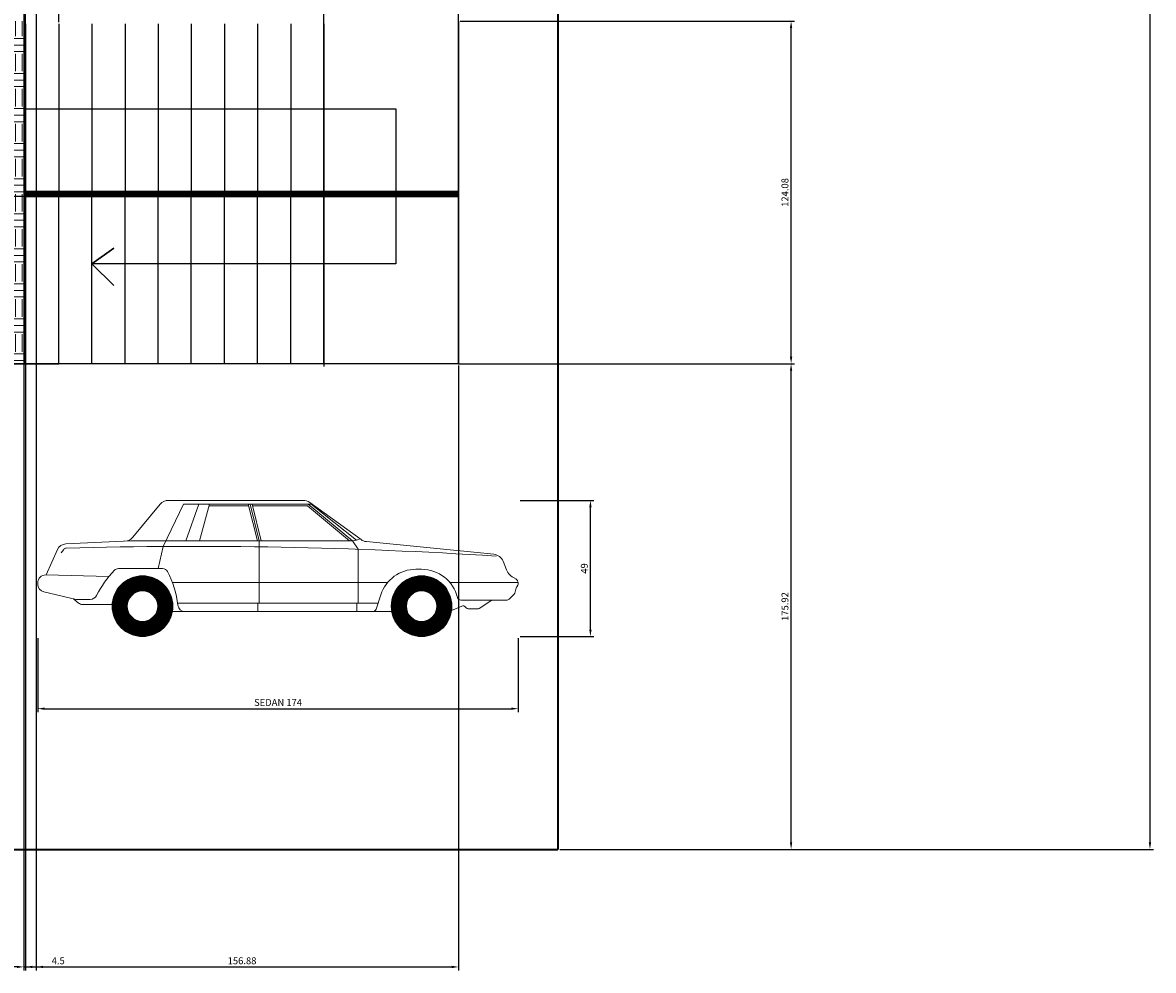
# Model space of a CAD drawing. Units: inches. Extents: x 204 to 942, y 1794 to 2670.
# Tile 2 of 6: x 533 to 942, y 1794 to 2138. Entities that reach past the tile are written whole.
import ezdxf

# ---------------------------------------------------------------- set-up
doc = ezdxf.new("R2010")
doc.units = ezdxf.units.IN
for name, color, linetype, lineweight in [('A-ANNO-DIMS', 2, 'Continuous', 18), ('A-FLOR-OTLN', 7, 'Continuous', 25), ('A-FLOR-STRS', 7, 'Continuous', 25), ('C-PRKG', 8, 'Continuous', 25), ('C-PRKG-VEHI', 8, 'Continuous', 18), ('C-PROP', 7, 'Continuous', 35)]:
    doc.layers.add(name, color=color, linetype=linetype, lineweight=lineweight)
doc.layers.add('A-FLOR-PATT', color=251, linetype='Continuous', lineweight=13, true_color=0x636466)
doc.styles.get("Standard").update_dxf_attribs({"font": 'arial.ttf'})
doc.dimstyles.new('ISO-25', dxfattribs={"dimtxt": 2.5, "dimasz": 2.5, "dimexe": 1.25, "dimexo": 0.625, "dimtad": 1, "dimtxsty": 'Standard', "dimcen": 2.5, "dimadec": 0, "dimazin": 0, "dimtfac": 1, "dimtmove": 0, "dimatfit": 3, "dimfxl": 1, "dimarcsym": 0})

# ---------------------------------------------------------------- blocks, each defined once
blk = doc.blocks.new('Car - sedan  side')
for p, q in [((-77.81, 49.34), (-126.58, 49.34)), ((-139.53, 35.99), (-129.64, 47.91)), ((-128.57, 32.64), (-121.22, 48.02)), ((-74.7, 48.02), (-121.22, 48.02)), ((-120.32, 34.67), (-115.67, 48.02)), ((-115.4, 34.67), (-111.74, 48.02)), ((-97.55, 47.3), (-111.94, 47.3)), ((-94.41, 34.67), (-97.73, 48.02)), ((-93.72, 34.67), (-97.04, 48.02)), ((-93.03, 34.67), (-96.34, 48.02)), ((-76.26, 47.3), (-96.16, 47.3)), ((-61.08, 34.66), (-76.26, 47.3)), ((-60.02, 34.65), (-76.07, 48.02)), ((-56.87, 35.13), (-75.48, 48.59)), ((-58.54, 34.93), (-74.99, 48.02)), ((-140.23, 34.67), (-163.88, 33.56)), ((-62.28, 34.67), (-140.23, 34.67)), ((-93.72, 19.62), (-93.72, 34.67)), ((-62.28, 34.67), (-60.02, 34.65)), ((-60.02, 34.65), (-58.54, 34.93)), ((-57.97, 31.61), (-60.02, 34.65)), ((-57.21, 35.38), (-58.54, 34.93)), ((-54.93, 34.4), (-8.75, 29.8)), ((-170.93, 22.32), (-166.81, 31.56)), ((-164.57, 31.6), (-165.48, 30.35)), ((-130.39, 24.63), (-128.57, 32.64)), ((-57.97, 19.62), (-57.97, 31.61)), ((-128.78, 24.63), (-144.79, 24.63)), ((-4.21, 24.18), (-5.42, 27.27)), ((-148.26, 21.7), (-171.11, 22.33)), ((-36.97, 24.38), (-34.94, 24.38)), ((-174, 19.51), (-174, 18.91)), ((-47.2, 19.62), (-125.23, 19.62)), ((-93.72, 12.14), (-93.72, 19.62)), ((-57.97, 12.14), (-57.97, 19.62)), ((0, 19.62), (-24.7, 19.62)), ((-160.12, 13.48), (-171.81, 16.16)), ((-159.22, 12.14), (-161.08, 13.7)), ((-155.01, 13.48), (-160.12, 13.48)), ((-51.4, 9.89), (-49.69, 15.14)), ((-4.23, 13.19), (-20.72, 13.19)), ((-9.5, 13.19), (-14.1, 10.2)), ((-3.22, 13.59), (-1.77, 14.97)), ((-147.03, 11.6), (-157.73, 11.6)), ((-120.62, 9.03), (-125.23, 9.03)), ((-50.67, 12.14), (-123.32, 12.14)), ((-45.76, 9.03), (-120.62, 9.03)), ((-94.21, 9.03), (-94.21, 12.14)), ((-58.39, 9.03), (-58.39, 12.14)), ((-20.36, 11.06), (-24.06, 9.44)), ((-18.83, 10.42), (-19.11, 10.76)), ((-14.68, 10.03), (-18.01, 10.03))]:
    blk.add_line(p, q)
at = {"const_width": 5.49}
for points in [[(-127.8, 11, -1), (-144.3, 11, -1)], [(-26.69, 11, -1), (-43.19, 11, -1)]]:
    blk.add_lwpolyline(points, format="xyb", close=True, dxfattribs=at)
for centre, radius in [((-136.05, 11), 11), ((-34.94, 11), 11), ((-136.05, 11), 5.51), ((-34.94, 11), 5.51)]:
    blk.add_circle(centre, radius)
for centre, radius, start, end in [((-126.58, 45.38), 3.97, 90, 140.3029), ((-77.81, 45.38), 3.97, 54.135, 90), ((-163.72, 30.18), 3.38, 92.6827, 155.9736), ((-142.58, 38.53), 3.97, 272.6827, 320.3029), ((-54.54, 38.35), 3.97, 234.135, 264.3123), ((-163.62, 30.91), 1.17, 91.491, 143.9553), ((-118.51, -1702.12), 1734.79, 86.34698, 91.49105), ((-9.15, 25.82), 4, 21.3107, 84.3123), ((-144.79, 22.64), 1.98, 90, 136.3964), ((-128.78, 22.64), 1.98, 28.1371, 90), ((-171.18, 19.51), 2.82, 88.4193, 180), ((-118.09, -2.78), 38.85, 136.3964, 152.9097), ((-157.14, 7.48), 34.14, 6.5135, 28.1371), ((-36.97, 11), 13.38, 90, 161.9732), ((-34.94, 11), 13.38, 13.5864, 90), ((0.9, 26.18), 5.49, 201.3107, 247.7048), ((-1.92, 19.3), 1.94, 325.3744, 67.7048), ((-171.18, 18.91), 2.82, 180, 257.0905), ((-3.82, 17.12), 2.96, 313.7173, 352.3839), ((2.46, 16.28), 3.37, 145.3744, 172.3839), ((-155.01, 16.1), 2.62, 270, 332.9097), ((-20.72, 14.43), 1.24, 193.5864, 270), ((-4.23, 14.65), 1.46, 270, 313.7173), ((-157.73, 13.93), 2.32, 230.1291, 270), ((-120.62, 11.65), 2.62, 186.5135, 270), ((-52.58, 10.27), 1.24, 270, 341.9732), ((-19.93, 10.09), 1.06, 39.301, 113.7159), ((-18.01, 11.09), 1.06, 219.301, 270), ((-14.68, 11.09), 1.06, 270, 303.047)]:
    blk.add_arc(centre, radius, start, end)
blk = doc.blocks.new('*D12')
at = {"layer": 'A-ANNO-DIMS', "color": 0, "lineweight": -2, "transparency": 16777216}
for p, q in [((727.37, 2624.26), (942.46, 2624.26)), ((941.21, 2621.76), (941.21, 1840.76)), ((727.37, 1838.26), (942.46, 1838.26))]:
    blk.add_line(p, q, dxfattribs=at)
at = {"layer": 'A-ANNO-DIMS', "color": 0, "transparency": 16777216}
for points in [[(940.79, 2621.76), (941.63, 2621.76), (941.21, 2624.26)], [(940.79, 1840.76), (941.63, 1840.76), (941.21, 1838.26)]]:
    blk.add_solid(points, dxfattribs=at)
at = {"layer": 'Defpoints', "color": 0, "transparency": 16777216}
for p in [(726.74, 2624.26), (726.74, 1838.26), (941.21, 1838.26)]:
    blk.add_point(p, dxfattribs=at)
at = {"layer": 'A-ANNO-DIMS', "color": 0, "transparency": 16777216, "insert": (939.31, 2231.26), "char_height": 2.5, "attachment_point": 5, "rotation": 90}
blk.add_mtext('786', dxfattribs=at)
blk = doc.blocks.new('*D36')
at = {"layer": 'A-ANNO-DIMS', "color": 0, "lineweight": -2, "transparency": 16777216}
for p, q in [((538.28, 1914.72), (538.28, 1887.97)), ((712.39, 1914.72), (712.39, 1887.97)), ((540.78, 1889.22), (709.89, 1889.22))]:
    blk.add_line(p, q, dxfattribs=at)
at = {"layer": 'A-ANNO-DIMS', "color": 0, "transparency": 16777216}
for points in [[(540.78, 1889.64), (540.78, 1888.81), (538.28, 1889.22)], [(709.89, 1889.64), (709.89, 1888.81), (712.39, 1889.22)]]:
    blk.add_solid(points, dxfattribs=at)
at = {"layer": 'Defpoints', "color": 0, "transparency": 16777216}
for p in [(538.28, 1915.34), (712.39, 1915.34), (712.39, 1889.22)]:
    blk.add_point(p, dxfattribs=at)
at = {"layer": 'A-ANNO-DIMS', "color": 0, "transparency": 16777216, "insert": (625.34, 1891.14), "char_height": 2.5, "attachment_point": 5}
blk.add_mtext('SEDAN 174', dxfattribs=at)
blk = doc.blocks.new('*D37')
at = {"layer": 'A-ANNO-DIMS', "color": 0, "lineweight": -2, "transparency": 16777216}
for p, q in [((713.02, 1964.69), (739.76, 1964.69)), ((738.51, 1917.84), (738.51, 1962.19)), ((713.02, 1915.34), (739.76, 1915.34))]:
    blk.add_line(p, q, dxfattribs=at)
at = {"layer": 'A-ANNO-DIMS', "color": 0, "transparency": 16777216}
for points in [[(738.1, 1962.19), (738.93, 1962.19), (738.51, 1964.69)], [(738.1, 1917.84), (738.93, 1917.84), (738.51, 1915.34)]]:
    blk.add_solid(points, dxfattribs=at)
at = {"layer": 'Defpoints', "color": 0, "transparency": 16777216}
for p in [(712.39, 1964.69), (738.51, 1964.69), (712.39, 1915.34)]:
    blk.add_point(p, dxfattribs=at)
at = {"layer": 'A-ANNO-DIMS', "color": 0, "transparency": 16777216, "insert": (736.61, 1940.01), "char_height": 2.5, "attachment_point": 5, "rotation": 90}
blk.add_mtext('49', dxfattribs=at)
blk = doc.blocks.new('*D43')
at = {"layer": 'A-ANNO-DIMS', "color": 0, "lineweight": -2, "transparency": 16777216}
for p, q in [((727.37, 2014.18), (812.46, 2014.18)), ((811.21, 1840.76), (811.21, 2011.68)), ((727.37, 1838.26), (812.46, 1838.26))]:
    blk.add_line(p, q, dxfattribs=at)
at = {"layer": 'A-ANNO-DIMS', "color": 0, "transparency": 16777216}
for points in [[(810.79, 2011.68), (811.62, 2011.68), (811.21, 2014.18)], [(810.79, 1840.76), (811.62, 1840.76), (811.21, 1838.26)]]:
    blk.add_solid(points, dxfattribs=at)
at = {"layer": 'Defpoints', "color": 0, "transparency": 16777216}
for p in [(726.74, 2014.18), (811.21, 2014.18), (726.74, 1838.26)]:
    blk.add_point(p, dxfattribs=at)
at = {"layer": 'A-ANNO-DIMS', "color": 0, "transparency": 16777216, "insert": (809.31, 1926.22), "char_height": 2.5, "attachment_point": 5, "rotation": 90}
blk.add_mtext('175.92', dxfattribs=at)
blk = doc.blocks.new('*D45')
at = {"layer": 'A-ANNO-DIMS', "color": 0, "lineweight": -2, "transparency": 16777216}
for p, q in [((691.37, 2138.26), (812.46, 2138.26)), ((811.21, 2016.68), (811.21, 2135.76)), ((691.37, 2014.18), (812.46, 2014.18))]:
    blk.add_line(p, q, dxfattribs=at)
at = {"layer": 'A-ANNO-DIMS', "color": 0, "transparency": 16777216}
for points in [[(810.79, 2135.76), (811.62, 2135.76), (811.21, 2138.26)], [(810.79, 2016.68), (811.62, 2016.68), (811.21, 2014.18)]]:
    blk.add_solid(points, dxfattribs=at)
at = {"layer": 'Defpoints', "color": 0, "transparency": 16777216}
for p in [(690.74, 2138.26), (811.21, 2138.26), (690.74, 2014.18)]:
    blk.add_point(p, dxfattribs=at)
at = {"layer": 'A-ANNO-DIMS', "color": 0, "transparency": 16777216, "insert": (809.31, 2076.22), "char_height": 2.5, "attachment_point": 5, "rotation": 90}
blk.add_mtext('124.08', dxfattribs=at)
blk = doc.blocks.new('*D46')
at = {"layer": 'A-ANNO-DIMS', "color": 0, "lineweight": -2, "transparency": 16777216}
for p, q in [((533.86, 2013.55), (533.86, 1794.41)), ((690.74, 2013.55), (690.74, 1794.41)), ((536.36, 1795.66), (688.24, 1795.66))]:
    blk.add_line(p, q, dxfattribs=at)
at = {"layer": 'A-ANNO-DIMS', "color": 0, "transparency": 16777216}
for points in [[(536.36, 1796.08), (536.36, 1795.24), (533.86, 1795.66)], [(688.24, 1796.08), (688.24, 1795.24), (690.74, 1795.66)]]:
    blk.add_solid(points, dxfattribs=at)
at = {"layer": 'Defpoints', "color": 0, "transparency": 16777216}
for p in [(533.86, 2014.18), (690.74, 2014.18), (690.74, 1795.66)]:
    blk.add_point(p, dxfattribs=at)
at = {"layer": 'A-ANNO-DIMS', "color": 0, "transparency": 16777216, "insert": (612.3, 1797.56), "char_height": 2.5, "attachment_point": 5}
blk.add_mtext('156.88', dxfattribs=at)
blk = doc.blocks.new('*D47')
at = {"layer": 'A-ANNO-DIMS', "color": 0, "lineweight": -2, "transparency": 16777216}
for p, q in [((533.86, 2137.88), (533.86, 2668.11)), ((536.36, 2666.86), (543.38, 2666.86)), ((545.88, 2137.88), (545.88, 2668.11))]:
    blk.add_line(p, q, dxfattribs=at)
at = {"layer": 'A-ANNO-DIMS', "color": 0, "transparency": 16777216}
for points in [[(536.36, 2667.28), (536.36, 2666.44), (533.86, 2666.86)], [(543.38, 2667.28), (543.38, 2666.44), (545.88, 2666.86)]]:
    blk.add_solid(points, dxfattribs=at)
at = {"layer": 'Defpoints', "color": 0, "transparency": 16777216}
for p in [(545.88, 2666.86), (533.86, 2137.26), (545.88, 2137.26)]:
    blk.add_point(p, dxfattribs=at)
at = {"layer": 'A-ANNO-DIMS', "color": 0, "transparency": 16777216, "insert": (539.87, 2668.76), "char_height": 2.5, "attachment_point": 5}
blk.add_mtext('12.012', dxfattribs=at)
blk = doc.blocks.new('*D48')
at = {"layer": 'A-ANNO-DIMS', "color": 0, "lineweight": -2, "transparency": 16777216}
for p, q in [((641.98, 2014.8), (641.98, 2668.11)), ((644.48, 2666.86), (688.24, 2666.86)), ((690.74, 2014.8), (690.74, 2668.11))]:
    blk.add_line(p, q, dxfattribs=at)
at = {"layer": 'A-ANNO-DIMS', "color": 0, "transparency": 16777216}
for points in [[(644.48, 2667.28), (644.48, 2666.44), (641.98, 2666.86)], [(688.24, 2667.28), (688.24, 2666.44), (690.74, 2666.86)]]:
    blk.add_solid(points, dxfattribs=at)
at = {"layer": 'Defpoints', "color": 0, "transparency": 16777216}
for p in [(690.74, 2666.86), (641.98, 2014.18), (690.74, 2014.18)]:
    blk.add_point(p, dxfattribs=at)
at = {"layer": 'A-ANNO-DIMS', "color": 0, "transparency": 16777216, "insert": (666.36, 2668.76), "char_height": 2.5, "attachment_point": 5}
blk.add_mtext('48.77', dxfattribs=at)
blk = doc.blocks.new('*D49')
at = {"layer": 'A-ANNO-DIMS', "color": 0, "lineweight": -2, "transparency": 16777216}
for p, q in [((533.24, 2074.72), (292.89, 2074.72)), ((294.14, 2016.68), (294.14, 2072.22)), ((533.24, 2014.18), (292.89, 2014.18))]:
    blk.add_line(p, q, dxfattribs=at)
at = {"layer": 'A-ANNO-DIMS', "color": 0, "transparency": 16777216}
for points in [[(293.73, 2072.22), (294.56, 2072.22), (294.14, 2074.72)], [(293.73, 2016.68), (294.56, 2016.68), (294.14, 2014.18)]]:
    blk.add_solid(points, dxfattribs=at)
at = {"layer": 'Defpoints', "color": 0, "transparency": 16777216}
for p in [(294.14, 2074.72), (533.86, 2074.72), (533.86, 2014.18)]:
    blk.add_point(p, dxfattribs=at)
at = {"layer": 'A-ANNO-DIMS', "color": 0, "transparency": 16777216, "insert": (292.24, 2044.45), "char_height": 2.5, "attachment_point": 5, "rotation": 90}
blk.add_mtext('60.54', dxfattribs=at)
blk = doc.blocks.new('*D50')
at = {"layer": 'A-ANNO-DIMS', "color": 0, "lineweight": -2, "transparency": 16777216}
for p, q in [((533.24, 2587.63), (533.24, 1794.41)), ((537.74, 2578.63), (537.74, 1794.41)), ((530.74, 1795.66), (528.24, 1795.66)), ((533.24, 1795.66), (537.74, 1795.66)), ((540.24, 1795.66), (548.67, 1795.66))]:
    blk.add_line(p, q, dxfattribs=at)
at = {"layer": 'A-ANNO-DIMS', "color": 0, "transparency": 16777216}
for points in [[(530.74, 1796.08), (530.74, 1795.24), (533.24, 1795.66)], [(540.24, 1796.08), (540.24, 1795.24), (537.74, 1795.66)]]:
    blk.add_solid(points, dxfattribs=at)
at = {"layer": 'Defpoints', "color": 0, "transparency": 16777216}
for p in [(533.24, 2588.26), (537.74, 2579.26), (537.74, 1795.66)]:
    blk.add_point(p, dxfattribs=at)
at = {"layer": 'A-ANNO-DIMS', "color": 0, "transparency": 16777216, "insert": (545.7, 1797.56), "char_height": 2.5, "attachment_point": 5}
blk.add_mtext('4.5', dxfattribs=at)

msp = doc.modelspace()

# ---------------------------------------------------------------- hatches: boundary and pattern name
at = {"layer": 'A-FLOR-PATT'}
h = msp.add_hatch(dxfattribs=at)
h.set_pattern_fill('EARTH', color=256)
h.paths.add_polyline_path([(533.8633, 2137.2597), (533.8633, 2138.2597), (473.5284, 2138.2597), (473.5284, 2138.2472), (471.5284, 2138.2472), (437.5284, 2138.2472), (372.7443, 2138.2597), (336.7443, 2138.2597), (336.7443, 2014.1774), (533.8633, 2014.1774)])

# ---------------------------------------------------------------- linework, layer by layer
at = {"layer": 'A-FLOR-OTLN'}
msp.add_line((336.7443, 2014.1774), (545.8757, 2014.1774), dxfattribs=at)
at = {"layer": 'A-FLOR-STRS'}
for p, q in [((533.8633, 2014.1774), (533.8633, 2138.2597)), ((533.8633, 2137.2597), (533.8633, 2013.1774)), ((533.8633, 2137.2597), (533.8633, 2075.7185)), ((545.8757, 2137.2597), (545.8757, 2075.7185)), ((557.8882, 2137.2597), (557.8882, 2075.7185)), ((569.9007, 2137.2597), (569.9007, 2075.7185)), ((581.9132, 2137.2597), (581.9132, 2075.7185)), ((593.9257, 2137.2597), (593.9257, 2075.7185)), ((605.9381, 2137.2597), (605.9381, 2075.7185)), ((617.9506, 2137.2597), (617.9506, 2075.7185)), ((629.9631, 2137.2597), (629.9631, 2075.7185)), ((641.9756, 2014.1774), (641.9756, 2138.2597)), ((641.9756, 2137.2597), (641.9756, 2013.1774)), ((641.9756, 2137.2597), (641.9756, 2075.7185)), ((690.7443, 2138.2597), (690.7443, 2014.1774)), ((533.8633, 2106.4891), (667.9618, 2106.4891)), ((667.9618, 2106.4891), (667.9618, 2050.3383)), ((533.8633, 2076.7185), (690.7443, 2076.7185)), ((533.8633, 2076.2185), (690.7443, 2076.2185)), ((533.8633, 2075.7185), (690.7443, 2075.7185)), ((533.8633, 2014.1774), (533.8633, 2075.7185)), ((533.8633, 2075.7185), (690.7443, 2075.7185)), ((533.8633, 2075.2185), (690.7443, 2075.2185)), ((533.8633, 2074.7185), (690.7443, 2074.7185)), ((545.8757, 2014.1774), (545.8757, 2075.7185)), ((557.8882, 2014.1774), (557.8882, 2075.7185)), ((569.9007, 2014.1774), (569.9007, 2075.7185)), ((581.9132, 2014.1774), (581.9132, 2075.7185)), ((593.9257, 2014.1774), (593.9257, 2075.7185)), ((605.9381, 2014.1774), (605.9381, 2075.7185)), ((617.9506, 2014.1774), (617.9506, 2075.7185)), ((629.9631, 2014.1774), (629.9631, 2075.7185)), ((641.9756, 2014.1774), (641.9756, 2075.7185)), ((690.7443, 2014.1774), (690.7443, 2075.7185)), ((557.8882, 2050.3383), (565.8504, 2056.0074)), ((565.8504, 2056.0074), (557.8882, 2050.3383)), ((569.9007, 2050.3383), (557.8882, 2050.3383)), ((557.8882, 2050.3383), (565.8504, 2042.5308)), ((667.9618, 2050.3383), (569.9007, 2050.3383)), ((690.7443, 2014.1774), (533.8633, 2014.1774)), ((690.7443, 2014.1774), (641.9756, 2014.1774))]:
    msp.add_line(p, q, dxfattribs=at)
at = {"layer": 'C-PRKG'}
msp.add_line((690.7443, 2014.1774), (726.7443, 2014.1774), dxfattribs=at)
at = {"layer": 'C-PROP'}
for p in [(726.7443, 2102.2597), (336.7443, 1838.2597)]:
    msp.add_line(p, (726.7443, 1838.2597), dxfattribs=at)
msp.add_lwpolyline([(336.7443, 2102.2597), (336.7443, 2624.2597), (726.7443, 2624.2597), (726.7443, 2102.2597)], dxfattribs=at)

# ---------------------------------------------------------------- block references
at = {"layer": 'C-PRKG-VEHI'}
msp.add_blockref('Car - sedan  side', (712.2811, 1915.3411), dxfattribs=at)

# ---------------------------------------------------------------- dimensions: what is measured, and where the dimension line sits
at = {"layer": 'A-ANNO-DIMS'}
for base, p1, p2, override, picture, middle in [((545.8757, 2666.8597), (533.8633, 2137.2597), (545.8757, 2137.2597), {"dimdec": 3, "dimlfac": 1, "dimrnd": 0, "dimzin": 0, "dimdsep": 46, "dimlunit": 2}, '*D47', (539.8695, 2668.7611)), ((690.7443, 2666.8597), (641.9756, 2014.1774), (690.7443, 2014.1774), {"dimdec": 2, "dimlfac": 1, "dimrnd": 0, "dimzin": 0, "dimdsep": 46, "dimlunit": 2}, '*D48', (666.3599, 2668.7611)), ((537.7443, 1795.6597), (533.2443, 2588.2597), (537.7443, 2579.2597), {"dimdec": 1, "dimlfac": 1, "dimrnd": 0, "dimzin": 0, "dimdsep": 46, "dimlunit": 2}, '*D50', (545.7047, 1797.556)), ((690.7443, 1795.6597), (533.8633, 2014.1774), (690.7443, 2014.1774), {"dimdec": 2, "dimlfac": 1, "dimrnd": 0, "dimzin": 0, "dimdsep": 46, "dimlunit": 2}, '*D46', (612.3038, 1797.5611))]:
    dim = msp.add_linear_dim(base=base, p1=p1, p2=p2, dimstyle='ISO-25', override=override, dxfattribs=at)
    dim.commit()
    dim.dimension.update_dxf_attribs({"geometry": picture, "text_midpoint": middle})
for base, p1, p2, override, picture, middle in [((941.2084, 1838.2597), (726.7443, 2624.2597), (726.7443, 1838.2597), {"dimclrd": 0, "dimclre": 0, "dimclrt": 0}, '*D12', (939.307, 2231.2597)), ((811.2079, 2138.2597), (690.7443, 2014.1774), (690.7443, 2138.2597), {"dimdec": 2, "dimlfac": 1, "dimrnd": 0, "dimzin": 0, "dimdsep": 46, "dimlunit": 2}, '*D45', (809.3064, 2076.2185)), ((294.1443, 2074.7185), (533.8633, 2014.1774), (533.8633, 2074.7185), {"dimdec": 2, "dimlfac": 1, "dimrnd": 0, "dimzin": 0, "dimdsep": 46, "dimlunit": 2}, '*D49', (292.2429, 2044.4479)), ((811.2079, 2014.1774), (726.7443, 1838.2597), (726.7443, 2014.1774), {"dimdec": 2, "dimlfac": 1, "dimrnd": 0, "dimzin": 0, "dimdsep": 46, "dimlunit": 2}, '*D43', (809.3064, 1926.2185)), ((738.5119, 1964.686), (712.3949, 1915.3411), (712.3949, 1964.686), {"dimdec": 0, "dimlfac": 1, "dimrnd": 0, "dimzin": 0, "dimdsep": 46, "dimlunit": 2}, '*D37', (736.6105, 1940.0135))]:
    dim = msp.add_linear_dim(base=base, p1=p1, p2=p2, angle=90, dimstyle='ISO-25', override=override, dxfattribs=at)
    dim.commit()
    dim.dimension.update_dxf_attribs({"geometry": picture, "text_midpoint": middle})
dim = msp.add_linear_dim(base=(712.3949, 1889.224), p1=(538.2811, 1915.3411), p2=(712.3949, 1915.3411), text='SEDAN <>', dimstyle='ISO-25', override={"dimdec": 0, "dimlfac": 1, "dimrnd": 0, "dimzin": 0, "dimdsep": 46, "dimlunit": 2}, dxfattribs=at)
dim.commit()
dim.dimension.update_dxf_attribs({"geometry": '*D36', "text_midpoint": (625.338, 1891.1416)})

doc.saveas('drawing.dxf')
